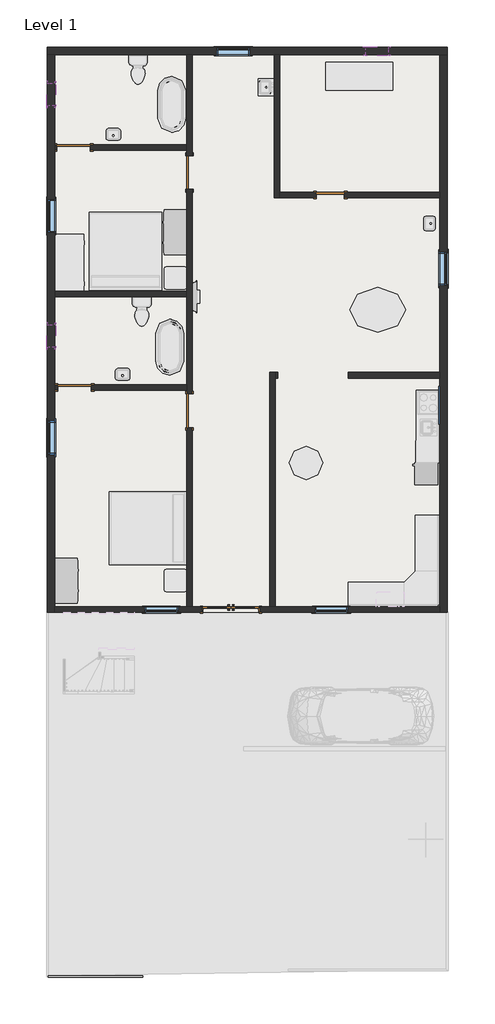
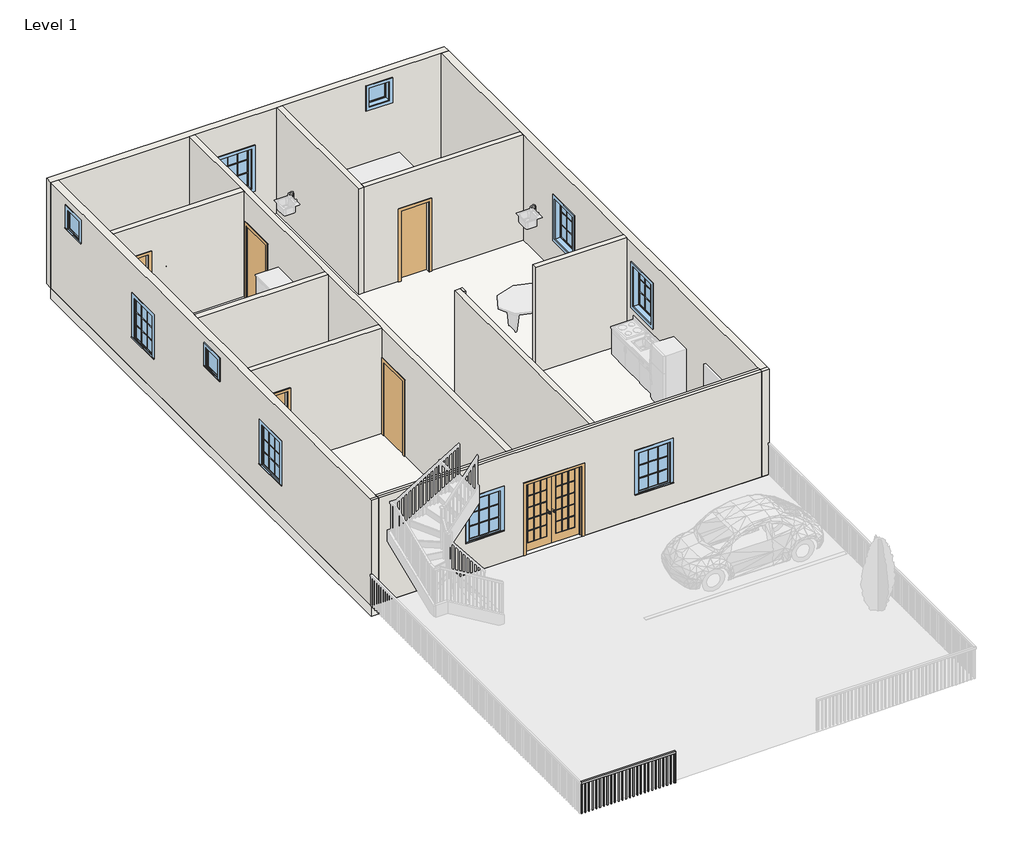
# One storey, part 1 of 5: 13 walls, 10 windows, 6 doors, 1 railing, 1 slab.
"""IFC4 building model written with IfcOpenShell, lengths in millimetres."""

from ifc_helpers import new_model, si_unit, frame, origin, origin_with_axes, place, context, project, spatial, polyline, outline, extrude, faceted_brep, transform, mapped, element, save
from components import door_31a77bde, door_255cab33, door_686f89d2, door_16372e1c, window_29c06734, window_5c190c7e, window_e41d21a6

model = new_model("IFC4")

# Units and contexts
model_context = context("Model", 3, world=origin())
ifc_project = project(units=[si_unit("LENGTHUNIT", "METRE", prefix="MILLI")], contexts=[model_context])

# Site, building, storey
site = spatial("IfcSite", under=ifc_project)
building = spatial("IfcBuilding", under=site)
storey = spatial("IfcBuildingStorey", under=building, Name="Level 1", Elevation=0.0)

# Doors
placement = place(None, origin())
door_shape = door_31a77bde(model_context)
element("IfcDoor", 1, ObjectType="Door-Interior-Double-Full Glass-Wood : 60\" x 80\"", at=placement, inside=storey, context=model_context, shape_type="MappedRepresentation", body=[
    mapped(door_shape, transform((-4021.3170266, -2394.0326646, 0.0), x_axis=(1.0, 0.0, 0.0), y_axis=(0.0, 1.0, 0.0), z_axis=(0.0, 0.0, 1.0))),
])
door_2_shape = door_255cab33(model_context)
element("IfcDoor", 2, ObjectType="Single-Flush : 30\" x 80\"", at=placement, inside=storey, context=model_context, shape_type="MappedRepresentation", body=[
    mapped(door_2_shape, transform((-1316.2170266, 8880.3923354, 0.0), x_axis=(-1.0, 0.0, 0.0), y_axis=(0.0, -1.0, 0.0), z_axis=(0.0, 0.0, 1.0))),
])
door_3_shape = door_686f89d2(model_context)
element("IfcDoor", 3, ObjectType="Single-Flush : 36\" x 84\"", at=placement, inside=storey, context=model_context, shape_type="MappedRepresentation", body=[
    mapped(door_3_shape, transform((-8301.2170266, 10175.7923354, 0.0), x_axis=(-1.0, 0.0, 0.0), y_axis=(0.0, -1.0, 0.0), z_axis=(0.0, 0.0, 1.0))),
])
element("IfcDoor", 4, ObjectType="Single-Flush : 36\" x 84\"", at=placement, inside=storey, context=model_context, shape_type="MappedRepresentation", body=[
    mapped(door_3_shape, transform((-8275.8170266, 3647.9923354, 0.0), x_axis=(-1.0, 0.0, 0.0), y_axis=(0.0, -1.0, 0.0), z_axis=(0.0, 0.0, 1.0))),
])
door_4_shape = door_16372e1c(model_context)
element("IfcDoor", 5, ObjectType="Single-Flush : 36\" x 84\"", at=placement, inside=storey, context=model_context, shape_type="MappedRepresentation", body=[
    mapped(door_4_shape, transform((-5151.6170266, 9489.9923354, 0.0), x_axis=(0.0, 1.0, 0.0), y_axis=(-1.0, 0.0, 0.0), z_axis=(0.0, 0.0, 1.0))),
])
element("IfcDoor", 6, ObjectType="Single-Flush : 36\" x 84\"", at=placement, inside=storey, context=model_context, shape_type="MappedRepresentation", body=[
    mapped(door_4_shape, transform((-5151.6170266, 3012.9923354, 0.0), x_axis=(0.0, 1.0, 0.0), y_axis=(-1.0, 0.0, 0.0), z_axis=(0.0, 0.0, 1.0))),
])

# Railing
element("IfcRailing", 7, ObjectType="Handrail - Rectangular", at=placement, inside=storey, context=model_context, shape_type="SweptSolid", body=[
    extrude(outline(polyline([(-8987.0170266, -12404.8076646), (-8987.0170266, -12354.0076646), (-6421.6170266, -12354.0076646), (-6421.6170266, -12404.8076646), (-8987.0170266, -12404.8076646)])), frame((0.0, 0.0, 863.6), z_axis=(0.0, 0.0, 1.0), x_axis=(1.0, 0.0, 0.0)), (0.0, 0.0, 1.0), 50.8),
    extrude(outline(polyline([(-6456.5420266, -12388.9326646), (-6456.5420266, -12369.8826646), (-6437.4920266, -12369.8826646), (-6437.4920266, -12388.9326646), (-6456.5420266, -12388.9326646)])), origin_with_axes(), (0.0, 0.0, 1.0), 863.6),
    extrude(outline(polyline([(-6558.1420266, -12388.9326646), (-6558.1420266, -12369.8826646), (-6539.0920266, -12369.8826646), (-6539.0920266, -12388.9326646), (-6558.1420266, -12388.9326646)])), origin_with_axes(), (0.0, 0.0, 1.0), 863.6),
    extrude(outline(polyline([(-6659.7420266, -12388.9326646), (-6659.7420266, -12369.8826646), (-6640.6920266, -12369.8826646), (-6640.6920266, -12388.9326646), (-6659.7420266, -12388.9326646)])), origin_with_axes(), (0.0, 0.0, 1.0), 863.6),
    extrude(outline(polyline([(-6761.3420266, -12388.9326646), (-6761.3420266, -12369.8826646), (-6742.2920266, -12369.8826646), (-6742.2920266, -12388.9326646), (-6761.3420266, -12388.9326646)])), origin_with_axes(), (0.0, 0.0, 1.0), 863.6),
    extrude(outline(polyline([(-6862.9420266, -12388.9326646), (-6862.9420266, -12369.8826646), (-6843.8920266, -12369.8826646), (-6843.8920266, -12388.9326646), (-6862.9420266, -12388.9326646)])), origin_with_axes(), (0.0, 0.0, 1.0), 863.6),
    extrude(outline(polyline([(-6964.5420266, -12388.9326646), (-6964.5420266, -12369.8826646), (-6945.4920266, -12369.8826646), (-6945.4920266, -12388.9326646), (-6964.5420266, -12388.9326646)])), origin_with_axes(), (0.0, 0.0, 1.0), 863.6),
    extrude(outline(polyline([(-7066.1420266, -12388.9326646), (-7066.1420266, -12369.8826646), (-7047.0920266, -12369.8826646), (-7047.0920266, -12388.9326646), (-7066.1420266, -12388.9326646)])), origin_with_axes(), (0.0, 0.0, 1.0), 863.6),
    extrude(outline(polyline([(-7167.7420266, -12388.9326646), (-7167.7420266, -12369.8826646), (-7148.6920266, -12369.8826646), (-7148.6920266, -12388.9326646), (-7167.7420266, -12388.9326646)])), origin_with_axes(), (0.0, 0.0, 1.0), 863.6),
    extrude(outline(polyline([(-7269.3420266, -12388.9326646), (-7269.3420266, -12369.8826646), (-7250.2920266, -12369.8826646), (-7250.2920266, -12388.9326646), (-7269.3420266, -12388.9326646)])), origin_with_axes(), (0.0, 0.0, 1.0), 863.6),
    extrude(outline(polyline([(-7370.9420266, -12388.9326646), (-7370.9420266, -12369.8826646), (-7351.8920266, -12369.8826646), (-7351.8920266, -12388.9326646), (-7370.9420266, -12388.9326646)])), origin_with_axes(), (0.0, 0.0, 1.0), 863.6),
    extrude(outline(polyline([(-7472.5420266, -12388.9326646), (-7472.5420266, -12369.8826646), (-7453.4920266, -12369.8826646), (-7453.4920266, -12388.9326646), (-7472.5420266, -12388.9326646)])), origin_with_axes(), (0.0, 0.0, 1.0), 863.6),
    extrude(outline(polyline([(-7574.1420266, -12388.9326646), (-7574.1420266, -12369.8826646), (-7555.0920266, -12369.8826646), (-7555.0920266, -12388.9326646), (-7574.1420266, -12388.9326646)])), origin_with_axes(), (0.0, 0.0, 1.0), 863.6),
    extrude(outline(polyline([(-7675.7420266, -12388.9326646), (-7675.7420266, -12369.8826646), (-7656.6920266, -12369.8826646), (-7656.6920266, -12388.9326646), (-7675.7420266, -12388.9326646)])), origin_with_axes(), (0.0, 0.0, 1.0), 863.6),
    extrude(outline(polyline([(-7777.3420266, -12388.9326646), (-7777.3420266, -12369.8826646), (-7758.2920266, -12369.8826646), (-7758.2920266, -12388.9326646), (-7777.3420266, -12388.9326646)])), origin_with_axes(), (0.0, 0.0, 1.0), 863.6),
    extrude(outline(polyline([(-7878.9420266, -12388.9326646), (-7878.9420266, -12369.8826646), (-7859.8920266, -12369.8826646), (-7859.8920266, -12388.9326646), (-7878.9420266, -12388.9326646)])), origin_with_axes(), (0.0, 0.0, 1.0), 863.6),
    extrude(outline(polyline([(-7980.5420266, -12388.9326646), (-7980.5420266, -12369.8826646), (-7961.4920266, -12369.8826646), (-7961.4920266, -12388.9326646), (-7980.5420266, -12388.9326646)])), origin_with_axes(), (0.0, 0.0, 1.0), 863.6),
    extrude(outline(polyline([(-8082.1420266, -12388.9326646), (-8082.1420266, -12369.8826646), (-8063.0920266, -12369.8826646), (-8063.0920266, -12388.9326646), (-8082.1420266, -12388.9326646)])), origin_with_axes(), (0.0, 0.0, 1.0), 863.6),
    extrude(outline(polyline([(-8183.7420266, -12388.9326646), (-8183.7420266, -12369.8826646), (-8164.6920266, -12369.8826646), (-8164.6920266, -12388.9326646), (-8183.7420266, -12388.9326646)])), origin_with_axes(), (0.0, 0.0, 1.0), 863.6),
    extrude(outline(polyline([(-8285.3420266, -12388.9326646), (-8285.3420266, -12369.8826646), (-8266.2920266, -12369.8826646), (-8266.2920266, -12388.9326646), (-8285.3420266, -12388.9326646)])), origin_with_axes(), (0.0, 0.0, 1.0), 863.6),
    extrude(outline(polyline([(-8386.9420266, -12388.9326646), (-8386.9420266, -12369.8826646), (-8367.8920266, -12369.8826646), (-8367.8920266, -12388.9326646), (-8386.9420266, -12388.9326646)])), origin_with_axes(), (0.0, 0.0, 1.0), 863.6),
    extrude(outline(polyline([(-8488.5420266, -12388.9326646), (-8488.5420266, -12369.8826646), (-8469.4920266, -12369.8826646), (-8469.4920266, -12388.9326646), (-8488.5420266, -12388.9326646)])), origin_with_axes(), (0.0, 0.0, 1.0), 863.6),
    extrude(outline(polyline([(-8590.1420266, -12388.9326646), (-8590.1420266, -12369.8826646), (-8571.0920266, -12369.8826646), (-8571.0920266, -12388.9326646), (-8590.1420266, -12388.9326646)])), origin_with_axes(), (0.0, 0.0, 1.0), 863.6),
    extrude(outline(polyline([(-8691.7420266, -12388.9326646), (-8691.7420266, -12369.8826646), (-8672.6920266, -12369.8826646), (-8672.6920266, -12388.9326646), (-8691.7420266, -12388.9326646)])), origin_with_axes(), (0.0, 0.0, 1.0), 863.6),
    extrude(outline(polyline([(-8793.3420266, -12388.9326646), (-8793.3420266, -12369.8826646), (-8774.2920266, -12369.8826646), (-8774.2920266, -12388.9326646), (-8793.3420266, -12388.9326646)])), origin_with_axes(), (0.0, 0.0, 1.0), 863.6),
    extrude(outline(polyline([(-8894.9420266, -12388.9326646), (-8894.9420266, -12369.8826646), (-8875.8920266, -12369.8826646), (-8875.8920266, -12388.9326646), (-8894.9420266, -12388.9326646)])), origin_with_axes(), (0.0, 0.0, 1.0), 863.6),
    extrude(outline(polyline([(-6440.6670266, -12388.9326646), (-6440.6670266, -12369.8826646), (-6421.6170266, -12369.8826646), (-6421.6170266, -12388.9326646), (-6440.6670266, -12388.9326646)])), origin_with_axes(), (0.0, 0.0, 1.0), 863.6),
    extrude(outline(polyline([(-8987.0170266, -12388.9326646), (-8987.0170266, -12369.8826646), (-8967.9670266, -12369.8826646), (-8967.9670266, -12388.9326646), (-8987.0170266, -12388.9326646)])), origin_with_axes(), (0.0, 0.0, 1.0), 863.6),
])

# Slab
element("IfcSlab", 8, ObjectType="Generic - 12\"", at=placement, inside=storey, context=model_context, shape_type="SweptSolid", body=[
    extrude(outline(polyline([(1858.7829734, 12690.3923354), (1858.7829734, -2473.4076646), (-9012.4170266, -2473.4076646), (-9012.4170266, 12690.3923354), (1858.7829734, 12690.3923354)])), frame((0.0, 0.0, -304.8), z_axis=(0.0, 0.0, 1.0), x_axis=(1.0, 0.0, 0.0)), (0.0, 0.0, 1.0), 304.8),
])

# Walls
element("IfcWall", 9, ObjectType="Generic - 8\"", at=placement, inside=storey, context=model_context, shape_type="Brep", body=[
    faceted_brep([(-9012.4170266, 12690.3923354, 0.0), (-8809.2170266, 12690.3923354, 0.0), (-5227.8170266, 12690.3923354, 0.0), (-5075.4170266, 12690.3923354, 0.0), (-2840.2170266, 12690.3923354, 0.0), (-2687.8170266, 12690.3923354, 0.0), (1655.5829734, 12690.3923354, 0.0), (1858.7829734, 12690.3923354, 0.0), (1858.7829734, 12690.3923354, 3048.0), (1655.5829734, 12690.3923354, 3048.0), (-2687.8170266, 12690.3923354, 3048.0), (-2840.2170266, 12690.3923354, 3048.0), (-5075.4170266, 12690.3923354, 3048.0), (-5227.8170266, 12690.3923354, 3048.0), (-8809.2170266, 12690.3923354, 3048.0), (-9012.4170266, 12690.3923354, 3048.0), (-3500.6170266, 12690.3923354, 2133.6), (-3500.6170266, 12690.3923354, 914.4), (-4415.0170266, 12690.3923354, 914.4), (-4415.0170266, 12690.3923354, 2133.6), (258.5829734, 12690.3923354, 2768.6), (258.5829734, 12690.3923354, 2159.0), (-351.0170266, 12690.3923354, 2159.0), (-351.0170266, 12690.3923354, 2768.6), (-9012.4170266, 12893.5923354, 0.0), (-9012.4170266, 12893.5923354, 3048.0), (1858.7829734, 12893.5923354, 3048.0), (1858.7829734, 12893.5923354, 0.0), (-3500.6170266, 12893.5923354, 2133.6), (-4415.0170266, 12893.5923354, 2133.6), (-4415.0170266, 12893.5923354, 914.4), (-3500.6170266, 12893.5923354, 914.4), (258.5829734, 12893.5923354, 2768.6), (-351.0170266, 12893.5923354, 2768.6), (-351.0170266, 12893.5923354, 2159.0), (258.5829734, 12893.5923354, 2159.0)], [[[0, 1, 2, 3, 4, 5, 6, 7, 8, 9, 10, 11, 12, 13, 14, 15], [16, 17, 18, 19], [20, 21, 22, 23]], [[24, 25, 26, 27], [28, 29, 30, 31], [32, 33, 34, 35]], [[7, 6, 5, 4, 3, 2, 1, 0, 24, 27]], [[0, 15, 25, 24]], [[8, 7, 27, 26]], [[17, 16, 28, 31]], [[18, 17, 31, 30]], [[19, 18, 30, 29]], [[16, 19, 29, 28]], [[21, 20, 32, 35]], [[22, 21, 35, 34]], [[23, 22, 34, 33]], [[20, 23, 33, 32]], [[15, 14, 13, 12, 11, 10, 9, 8, 26, 25]]]),
])
element("IfcWall", 10, ObjectType="Generic - 8\"", at=placement, inside=storey, context=model_context, shape_type="Brep", body=[
    faceted_brep([(-9012.4170266, 12690.3923354, 0.0), (-9012.4170266, -2473.4076646, 0.0), (-9012.4170266, -2473.4076646, 3048.0), (-9012.4170266, -2397.2076646, 3048.0), (-9012.4170266, 12690.3923354, 3048.0), (-9012.4170266, 8766.0923354, 2133.6), (-9012.4170266, 7851.6923354, 2133.6), (-9012.4170266, 7851.6923354, 914.4), (-9012.4170266, 8766.0923354, 914.4), (-9012.4170266, 2733.5923354, 2133.6), (-9012.4170266, 1819.1923354, 2133.6), (-9012.4170266, 1819.1923354, 914.4), (-9012.4170266, 2733.5923354, 914.4), (-9012.4170266, 11915.6923354, 2768.6), (-9012.4170266, 11306.0923354, 2768.6), (-9012.4170266, 11306.0923354, 2159.0), (-9012.4170266, 11915.6923354, 2159.0), (-9012.4170266, 5349.7923354, 2768.6), (-9012.4170266, 4740.1923354, 2768.6), (-9012.4170266, 4740.1923354, 2159.0), (-9012.4170266, 5349.7923354, 2159.0), (-8809.2170266, 12690.3923354, 0.0), (-8809.2170266, 12690.3923354, 3048.0), (-8809.2170266, 10251.9923354, 3048.0), (-8809.2170266, 10099.5923354, 3048.0), (-8809.2170266, 6264.1923354, 3048.0), (-8809.2170266, 6111.7923354, 3048.0), (-8809.2170266, 3724.1923354, 3048.0), (-8809.2170266, 3571.7923354, 3048.0), (-8809.2170266, -2321.0076646, 3048.0), (-8809.2170266, -2397.2076646, 3048.0), (-8809.2170266, -2473.4076646, 3048.0), (-8809.2170266, -2473.4076646, 0.0), (-8809.2170266, -2321.0076646, 0.0), (-8809.2170266, 3571.7923354, 0.0), (-8809.2170266, 3724.1923354, 0.0), (-8809.2170266, 6111.7923354, 0.0), (-8809.2170266, 6264.1923354, 0.0), (-8809.2170266, 10099.5923354, 0.0), (-8809.2170266, 10251.9923354, 0.0), (-8809.2170266, 8766.0923354, 2133.6), (-8809.2170266, 8766.0923354, 914.4), (-8809.2170266, 7851.6923354, 914.4), (-8809.2170266, 7851.6923354, 2133.6), (-8809.2170266, 2733.5923354, 2133.6), (-8809.2170266, 2733.5923354, 914.4), (-8809.2170266, 1819.1923354, 914.4), (-8809.2170266, 1819.1923354, 2133.6), (-8809.2170266, 11915.6923354, 2768.6), (-8809.2170266, 11915.6923354, 2159.0), (-8809.2170266, 11306.0923354, 2159.0), (-8809.2170266, 11306.0923354, 2768.6), (-8809.2170266, 5349.7923354, 2768.6), (-8809.2170266, 5349.7923354, 2159.0), (-8809.2170266, 4740.1923354, 2159.0), (-8809.2170266, 4740.1923354, 2768.6)], [[[0, 1, 2, 3, 4], [5, 6, 7, 8], [9, 10, 11, 12], [13, 14, 15, 16], [17, 18, 19, 20]], [[21, 22, 23, 24, 25, 26, 27, 28, 29, 30, 31, 32, 33, 34, 35, 36, 37, 38, 39], [40, 41, 42, 43], [44, 45, 46, 47], [48, 49, 50, 51], [52, 53, 54, 55]], [[1, 0, 21, 39, 38, 37, 36, 35, 34, 33, 32]], [[0, 4, 22, 21]], [[41, 40, 5, 8]], [[42, 41, 8, 7]], [[43, 42, 7, 6]], [[40, 43, 6, 5]], [[45, 44, 9, 12]], [[46, 45, 12, 11]], [[47, 46, 11, 10]], [[44, 47, 10, 9]], [[49, 48, 13, 16]], [[50, 49, 16, 15]], [[51, 50, 15, 14]], [[48, 51, 14, 13]], [[53, 52, 17, 20]], [[54, 53, 20, 19]], [[55, 54, 19, 18]], [[52, 55, 18, 17]], [[2, 1, 32, 31]], [[3, 2, 31, 30]], [[4, 3, 30, 29, 28, 27, 26, 25, 24, 23, 22]]]),
])
element("IfcWall", 11, ObjectType="Generic - 8\"", at=placement, inside=storey, context=model_context, shape_type="Brep", body=[
    faceted_brep([(1858.7829734, -2473.4076646, 0.0), (1858.7829734, 12690.3923354, 0.0), (1858.7829734, 12690.3923354, 3048.0), (1858.7829734, -2397.2076646, 3048.0), (1858.7829734, -2473.4076646, 3048.0), (1858.7829734, 2708.1923354, 2438.4), (1858.7829734, 3622.5923354, 2438.4), (1858.7829734, 3622.5923354, 1219.2), (1858.7829734, 2708.1923354, 1219.2), (1858.7829734, 6416.5923354, 2133.6), (1858.7829734, 7330.9923354, 2133.6), (1858.7829734, 7330.9923354, 914.4), (1858.7829734, 6416.5923354, 914.4), (1655.5829734, -2473.4076646, 0.0), (1655.5829734, -2473.4076646, 3048.0), (1655.5829734, -2397.2076646, 3048.0), (1655.5829734, -2321.0076646, 3048.0), (1655.5829734, 3901.9923354, 3048.0), (1655.5829734, 4054.3923354, 3048.0), (1655.5829734, 8804.1923354, 3048.0), (1655.5829734, 8956.5923354, 3048.0), (1655.5829734, 12690.3923354, 3048.0), (1655.5829734, 12690.3923354, 0.0), (1655.5829734, 8956.5923354, 0.0), (1655.5829734, 8804.1923354, 0.0), (1655.5829734, 4054.3923354, 0.0), (1655.5829734, 3901.9923354, 0.0), (1655.5829734, -2321.0076646, 0.0), (1655.5829734, 2708.1923354, 2438.4), (1655.5829734, 2708.1923354, 1219.2), (1655.5829734, 3622.5923354, 1219.2), (1655.5829734, 3622.5923354, 2438.4), (1655.5829734, 6416.5923354, 2133.6), (1655.5829734, 6416.5923354, 914.4), (1655.5829734, 7330.9923354, 914.4), (1655.5829734, 7330.9923354, 2133.6)], [[[0, 1, 2, 3, 4], [5, 6, 7, 8], [9, 10, 11, 12]], [[13, 14, 15, 16, 17, 18, 19, 20, 21, 22, 23, 24, 25, 26, 27], [28, 29, 30, 31], [32, 33, 34, 35]], [[1, 0, 13, 27, 26, 25, 24, 23, 22]], [[2, 1, 22, 21]], [[28, 31, 6, 5]], [[31, 30, 7, 6]], [[30, 29, 8, 7]], [[29, 28, 5, 8]], [[32, 35, 10, 9]], [[35, 34, 11, 10]], [[34, 33, 12, 11]], [[33, 32, 9, 12]], [[0, 4, 14, 13]], [[4, 3, 15, 14]], [[3, 2, 21, 20, 19, 18, 17, 16, 15]]]),
])
element("IfcWall", 12, ObjectType="INNER WALL 6\"", at=placement, inside=storey, context=model_context, shape_type="Brep", body=[
    faceted_brep([(-5227.8170266, 9032.7923354, 0.0), (-5227.8170266, 6264.1923354, 0.0), (-5227.8170266, 6111.7923354, 0.0), (-5227.8170266, 3724.1923354, 0.0), (-5227.8170266, 3571.7923354, 0.0), (-5227.8170266, 3470.1923354, 0.0), (-5227.8170266, 3470.1923354, 2133.6), (-5227.8170266, 2555.7923354, 2133.6), (-5227.8170266, 2555.7923354, 0.0), (-5227.8170266, -2321.0076646, 0.0), (-5227.8170266, -2321.0076646, 3048.0), (-5227.8170266, 3571.7923354, 3048.0), (-5227.8170266, 3724.1923354, 3048.0), (-5227.8170266, 6111.7923354, 3048.0), (-5227.8170266, 6264.1923354, 3048.0), (-5227.8170266, 10099.5923354, 3048.0), (-5227.8170266, 10251.9923354, 3048.0), (-5227.8170266, 12690.3923354, 3048.0), (-5227.8170266, 12690.3923354, 0.0), (-5227.8170266, 10251.9923354, 0.0), (-5227.8170266, 10099.5923354, 0.0), (-5227.8170266, 9947.1923354, 0.0), (-5227.8170266, 9947.1923354, 2133.6), (-5227.8170266, 9032.7923354, 2133.6), (-5075.4170266, 3470.1923354, 2133.6), (-5075.4170266, 3470.1923354, 0.0), (-5075.4170266, 9032.7923354, 0.0), (-5075.4170266, 9032.7923354, 2133.6), (-5075.4170266, 9947.1923354, 2133.6), (-5075.4170266, 9947.1923354, 0.0), (-5075.4170266, 12690.3923354, 0.0), (-5075.4170266, 12690.3923354, 3048.0), (-5075.4170266, -2321.0076646, 3048.0), (-5075.4170266, -2321.0076646, 0.0), (-5075.4170266, 2555.7923354, 0.0), (-5075.4170266, 2555.7923354, 2133.6)], [[[0, 1, 2, 3, 4, 5, 6, 7, 8, 9, 10, 11, 12, 13, 14, 15, 16, 17, 18, 19, 20, 21, 22, 23]], [[24, 25, 26, 27, 28, 29, 30, 31, 32, 33, 34, 35]], [[30, 29, 21, 20, 19, 18]], [[34, 33, 9, 8]], [[26, 25, 5, 4, 3, 2, 1, 0]], [[18, 17, 31, 30]], [[10, 9, 33, 32]], [[22, 21, 29, 28]], [[23, 22, 28, 27]], [[0, 23, 27, 26]], [[6, 5, 25, 24]], [[7, 6, 24, 35]], [[8, 7, 35, 34]], [[17, 16, 15, 14, 13, 12, 11, 10, 32, 31]]]),
])
element("IfcWall", 13, ObjectType="INNER WALL 6\"", at=placement, inside=storey, context=model_context, shape_type="Brep", body=[
    faceted_brep([(1655.5829734, -2321.0076646, 3048.0), (1655.5829734, -2321.0076646, 0.0), (-2814.8170266, -2321.0076646, 0.0), (-2967.2170266, -2321.0076646, 0.0), (-3233.9170266, -2321.0076646, 0.0), (-3233.9170266, -2321.0076646, 2057.4), (-4808.7170266, -2321.0076646, 2057.4), (-4808.7170266, -2321.0076646, 0.0), (-5075.4170266, -2321.0076646, 0.0), (-5227.8170266, -2321.0076646, 0.0), (-8809.2170266, -2321.0076646, 0.0), (-8809.2170266, -2321.0076646, 3048.0), (-5227.8170266, -2321.0076646, 3048.0), (-5075.4170266, -2321.0076646, 3048.0), (-2967.2170266, -2321.0076646, 3048.0), (-2814.8170266, -2321.0076646, 3048.0), (-6370.8170266, -2321.0076646, 2133.6), (-6370.8170266, -2321.0076646, 914.4), (-5456.4170266, -2321.0076646, 914.4), (-5456.4170266, -2321.0076646, 2133.6), (-1748.0170266, -2321.0076646, 1905.0), (-1748.0170266, -2321.0076646, 685.8), (-833.6170266, -2321.0076646, 685.8), (-833.6170266, -2321.0076646, 1905.0), (1655.5829734, -2473.4076646, 3048.0), (-8809.2170266, -2473.4076646, 3048.0), (-8809.2170266, -2473.4076646, 0.0), (-4808.7170266, -2473.4076646, 0.0), (-4808.7170266, -2473.4076646, 2057.4), (-3233.9170266, -2473.4076646, 2057.4), (-3233.9170266, -2473.4076646, 0.0), (1655.5829734, -2473.4076646, 0.0), (-6370.8170266, -2473.4076646, 2133.6), (-5456.4170266, -2473.4076646, 2133.6), (-5456.4170266, -2473.4076646, 914.4), (-6370.8170266, -2473.4076646, 914.4), (-1748.0170266, -2473.4076646, 1905.0), (-833.6170266, -2473.4076646, 1905.0), (-833.6170266, -2473.4076646, 685.8), (-1748.0170266, -2473.4076646, 685.8), (1655.5829734, -2397.2076646, 3048.0), (-8809.2170266, -2397.2076646, 3048.0)], [[[0, 1, 2, 3, 4, 5, 6, 7, 8, 9, 10, 11, 12, 13, 14, 15], [16, 17, 18, 19], [20, 21, 22, 23]], [[24, 25, 26, 27, 28, 29, 30, 31], [32, 33, 34, 35], [36, 37, 38, 39]], [[1, 31, 30, 4, 3, 2]], [[26, 10, 9, 8, 7, 27]], [[29, 5, 4, 30]], [[5, 29, 28, 6]], [[6, 28, 27, 7]], [[17, 16, 32, 35]], [[18, 17, 35, 34]], [[19, 18, 34, 33]], [[16, 19, 33, 32]], [[21, 20, 36, 39]], [[22, 21, 39, 38]], [[23, 22, 38, 37]], [[20, 23, 37, 36]], [[1, 0, 40, 24, 31]], [[11, 10, 26, 25, 41]], [[25, 24, 40, 41]], [[0, 15, 14, 13, 12, 11, 41, 40]]]),
])
element("IfcWall", 14, ObjectType="INNER WALL 6\"", at=placement, inside=storey, context=model_context, shape_type="Brep", body=[
    faceted_brep([(-2814.8170266, -2321.0076646, 0.0), (-2814.8170266, 3901.9923354, 0.0), (-2814.8170266, 4054.3923354, 0.0), (-2814.8170266, 4054.3923354, 3048.0), (-2814.8170266, 3901.9923354, 3048.0), (-2814.8170266, -2321.0076646, 3048.0), (-2967.2170266, -2321.0076646, 0.0), (-2967.2170266, -2321.0076646, 3048.0), (-2967.2170266, 4054.3923354, 3048.0), (-2967.2170266, 4054.3923354, 0.0)], [[[0, 1, 2, 3, 4, 5]], [[6, 7, 8, 9]], [[2, 1, 0, 6, 9]], [[0, 5, 7, 6]], [[3, 2, 9, 8]], [[5, 4, 3, 8, 7]]]),
])
element("IfcWall", 15, ObjectType="INNER WALL 6\"", at=placement, inside=storey, context=model_context, shape_type="SweptSolid", body=[
    extrude(outline(polyline([(-2751.3170266, 3901.9923354), (-2814.8170266, 3901.9923354), (-2814.8170266, 4054.3923354), (-2751.3170266, 4054.3923354), (-2751.3170266, 3901.9923354)])), origin_with_axes(), (0.0, 0.0, 1.0), 3048.0),
])
element("IfcWall", 16, ObjectType="INNER WALL 6\"", at=placement, inside=storey, context=model_context, shape_type="Brep", body=[
    faceted_brep([(-2840.2170266, 12690.3923354, 0.0), (-2840.2170266, 8804.1923354, 0.0), (-2840.2170266, 8804.1923354, 3048.0), (-2840.2170266, 12690.3923354, 3048.0), (-2687.8170266, 12690.3923354, 0.0), (-2687.8170266, 12690.3923354, 3048.0), (-2687.8170266, 8956.5923354, 3048.0), (-2687.8170266, 8804.1923354, 3048.0), (-2687.8170266, 8804.1923354, 0.0), (-2687.8170266, 8956.5923354, 0.0)], [[[0, 1, 2, 3]], [[4, 5, 6, 7, 8, 9]], [[1, 0, 4, 9, 8]], [[0, 3, 5, 4]], [[2, 1, 8, 7]], [[3, 2, 7, 6, 5]]]),
])
element("IfcWall", 17, ObjectType="INNER WALL 6\"", at=placement, inside=storey, context=model_context, shape_type="SweptSolid", body=[
    extrude(outline(polyline([(0.0, -2687.8170266), (0.0, -1697.2170266), (2032.0, -1697.2170266), (2032.0, -935.2170266), (0.0, -935.2170266), (0.0, 1655.5829734), (3048.0, 1655.5829734), (3048.0, -2687.8170266), (0.0, -2687.8170266)])), frame((0.0, 8804.1923354, 0.0), z_axis=(0.0, 1.0, 0.0), x_axis=(0.0, 0.0, 1.0)), (0.0, 0.0, 1.0), 152.4),
])
element("IfcWall", 18, ObjectType="INNER WALL 6\"", at=placement, inside=storey, context=model_context, shape_type="SweptSolid", body=[
    extrude(outline(polyline([(0.0, -8809.2170266), (0.0, -8758.4170266), (2133.6, -8758.4170266), (2133.6, -7844.0170266), (0.0, -7844.0170266), (0.0, -5227.8170266), (3048.0, -5227.8170266), (3048.0, -8809.2170266), (0.0, -8809.2170266)])), frame((0.0, 10099.5923354, 0.0), z_axis=(0.0, 1.0, 0.0), x_axis=(0.0, 0.0, 1.0)), (0.0, 0.0, 1.0), 152.4),
])
element("IfcWall", 19, ObjectType="INNER WALL 6\"", at=placement, inside=storey, context=model_context, shape_type="SweptSolid", body=[
    extrude(outline(polyline([(-5227.8170266, 6111.7923354), (-8809.2170266, 6111.7923354), (-8809.2170266, 6264.1923354), (-5227.8170266, 6264.1923354), (-5227.8170266, 6111.7923354)])), origin_with_axes(), (0.0, 0.0, 1.0), 3048.0),
])
element("IfcWall", 20, ObjectType="INNER WALL 6\"", at=placement, inside=storey, context=model_context, shape_type="SweptSolid", body=[
    extrude(outline(polyline([(0.0, -8809.2170266), (0.0, -8733.0170266), (2133.6, -8733.0170266), (2133.6, -7818.6170266), (0.0, -7818.6170266), (0.0, -5227.8170266), (3048.0, -5227.8170266), (3048.0, -8809.2170266), (0.0, -8809.2170266)])), frame((0.0, 3571.7923354, 0.0), z_axis=(0.0, 1.0, 0.0), x_axis=(0.0, 0.0, 1.0)), (0.0, 0.0, 1.0), 152.4),
])
element("IfcWall", 21, ObjectType="INNER WALL 6\"", at=placement, inside=storey, context=model_context, shape_type="SweptSolid", body=[
    extrude(outline(polyline([(1655.5829734, 3901.9923354), (-833.6170266, 3901.9923354), (-833.6170266, 4054.3923354), (1655.5829734, 4054.3923354), (1655.5829734, 3901.9923354)])), origin_with_axes(), (0.0, 0.0, 1.0), 3048.0),
])

# Windows
window_shape = window_29c06734(model_context)
element("IfcWindow", 22, ObjectType="Casement 3x3 with Trim : 36\" x 48\"", at=placement, inside=storey, context=model_context, shape_type="MappedRepresentation", body=[
    mapped(window_shape, transform((-8910.8170266, 8308.8923354, 0.0), x_axis=(0.0, 1.0, 0.0), y_axis=(-1.0, 0.0, 0.0), z_axis=(0.0, 0.0, 1.0))),
])
element("IfcWindow", 23, ObjectType="Casement 3x3 with Trim : 36\" x 48\"", at=placement, inside=storey, context=model_context, shape_type="MappedRepresentation", body=[
    mapped(window_shape, transform((-8910.8170266, 2276.3923354, 0.0), x_axis=(0.0, 1.0, 0.0), y_axis=(-1.0, 0.0, 0.0), z_axis=(0.0, 0.0, 1.0))),
])
element("IfcWindow", 24, ObjectType="Casement 3x3 with Trim : 36\" x 48\"", at=placement, inside=storey, context=model_context, shape_type="MappedRepresentation", body=[
    mapped(window_shape, transform((1757.1829734, 3165.3923354, 304.8), x_axis=(0.0, -1.0, 0.0), y_axis=(1.0, 0.0, 0.0), z_axis=(0.0, 0.0, 1.0))),
])
element("IfcWindow", 25, ObjectType="Casement 3x3 with Trim : 36\" x 48\"", at=placement, inside=storey, context=model_context, shape_type="MappedRepresentation", body=[
    mapped(window_shape, transform((1757.1829734, 6873.7923354, 0.0), x_axis=(0.0, -1.0, 0.0), y_axis=(1.0, 0.0, 0.0), z_axis=(0.0, 0.0, 1.0))),
])
element("IfcWindow", 26, ObjectType="Casement 3x3 with Trim : 36\" x 48\"", at=placement, inside=storey, context=model_context, shape_type="MappedRepresentation", body=[
    mapped(window_shape, transform((-3957.8170266, 12791.9923354, 0.0), x_axis=(1.0, 0.0, 0.0), y_axis=(0.0, 1.0, 0.0), z_axis=(0.0, 0.0, 1.0))),
])
window_2_shape = window_5c190c7e(model_context)
element("IfcWindow", 27, ObjectType="Casement 3x3 with Trim : 36\" x 48\"", at=placement, inside=storey, context=model_context, shape_type="MappedRepresentation", body=[
    mapped(window_2_shape, transform((-5913.6170266, -2397.2076646, 0.0), x_axis=(-1.0, 0.0, 0.0), y_axis=(0.0, -1.0, 0.0), z_axis=(0.0, 0.0, 1.0))),
])
element("IfcWindow", 28, ObjectType="Casement 3x3 with Trim : 36\" x 48\"", at=placement, inside=storey, context=model_context, shape_type="MappedRepresentation", body=[
    mapped(window_2_shape, transform((-1290.8170266, -2397.2076646, -228.6), x_axis=(-1.0, 0.0, 0.0), y_axis=(0.0, -1.0, 0.0), z_axis=(0.0, 0.0, 1.0))),
])
window_3_shape = window_e41d21a6(model_context)
element("IfcWindow", 29, ObjectType="Transom with Trim : 24\" x 24\"", at=placement, inside=storey, context=model_context, shape_type="MappedRepresentation", body=[
    mapped(window_3_shape, transform((-8910.8170266, 11648.9923354, 0.0), x_axis=(0.0, 1.0, 0.0), y_axis=(-1.0, 0.0, 0.0), z_axis=(0.0, 0.0, 1.0))),
])
element("IfcWindow", 30, ObjectType="Transom with Trim : 24\" x 24\"", at=placement, inside=storey, context=model_context, shape_type="MappedRepresentation", body=[
    mapped(window_3_shape, transform((-8910.8170266, 5083.0923354, 0.0), x_axis=(0.0, 1.0, 0.0), y_axis=(-1.0, 0.0, 0.0), z_axis=(0.0, 0.0, 1.0))),
])
element("IfcWindow", 31, ObjectType="Transom with Trim : 24\" x 24\"", at=placement, inside=storey, context=model_context, shape_type="MappedRepresentation", body=[
    mapped(window_3_shape, transform((-8.1170266, 12791.9923354, 0.0), x_axis=(1.0, 0.0, 0.0), y_axis=(0.0, 1.0, 0.0), z_axis=(0.0, 0.0, 1.0))),
])

save(model, "model.ifc")

# Revit data of these elements
# Type "Door-Interior-Double-Full Glass-Wood : 60\" x 80\""
#   Type Mark = "8"
#   Assembly Code = "C1020300"
#   Analytic Construction = "French door, wood frame with single glass"
#   Top Rail = 0' - 4 11/16"
#   Thickness = 0' - 1 3/8"
#   Thermal Resistance (R) = 1.0696 (h·ft²·°F)/BTU
#   Swing Angle [instance default] = 90.00°
#   Stiles = 0' - 4 3/4"
#   Rough Width = 5' - 2"
#   Rough Height = 6' - 9"
#   Panel Width = 2' - 6"
#   Height = 6' - 8"
#   Width = 5' - 0"
#   Heat Transfer Coefficient (U) = 0.9350 BTU/(h·ft²·°F)
#   Bottom Rail = 0' - 9 1/8"
#   Show Grill [instance default] = yes
#   Trim Material = Cherry
#   Panel Material = Cherry
#   Frame Material = Cherry
#   Door Handle Material = Aluminum
#   Visual Light Transmittance = 0
#   Solar Heat Gain Coefficient = 0
#   Wall Closure = (empty or 0)
#   Function = (empty or 0)
# Type "Single-Flush : 30\" x 80\""
#   Type Mark = "5"
#   Construction Type Id = "MDOOR"
#   Assembly Code = "C1020"
#   Analytic Construction = "Metal"
#   Thickness = 0' - 2"
#   Heat Transfer Coefficient (U) = 0.651978 BTU/(h·ft²·°F)
#   Height = 6' - 8"
#   Trim Projection Ext = 0' - 1"
#   Trim Projection Int = 0' - 1"
#   Trim Width = 0' - 3"
#   Width = 2' - 6"
#   Define Thermal Properties by = 1
#   Door Material = Door - Panel
#   Frame Material = Door - Frame
#   Visual Light Transmittance = 0
#   Solar Heat Gain Coefficient = 0
#   Function = (empty or 0)
#   Wall Closure = (empty or 0)
# Type "Single-Flush : 36\" x 84\""
#   Type Mark = "1"
#   Construction Type Id = "MDOOR"
#   Assembly Code = "C1020"
#   Analytic Construction = "Metal"
#   Thickness = 0' - 2"
#   Heat Transfer Coefficient (U) = 0.651978 BTU/(h·ft²·°F)
#   Height = 7' - 0"
#   Trim Projection Ext = 0' - 1"
#   Trim Projection Int = 0' - 1"
#   Trim Width = 0' - 3"
#   Width = 3' - 0"
#   Define Thermal Properties by = 1
#   Door Material = Door - Panel
#   Frame Material = Door - Frame
#   Visual Light Transmittance = 0
#   Solar Heat Gain Coefficient = 0
#   Function = (empty or 0)
#   Wall Closure = (empty or 0)
# Type "Handrail - Rectangular"
#   Assembly Code = "C2010400"
#   built-in parameter 1008612 = 0.0416667 (stored number, unit not read)
#   built-in parameter 1008611 = 0.0416667 (stored number, unit not read)
#   built-in parameter 1008609 = 0.333333 (stored number, unit not read)
#   built-in parameter 1008604 = 0.166667 (stored number, unit not read)
#   built-in parameter 1008603 = 0.166667 (stored number, unit not read)
#   Railing Height = 3' - 0"
#   built-in parameter 1008630 = 2
#   built-in parameter 1008610 = 2
#   built-in parameter 1008618 = Baluster - Square : 3/4"
# Type "Generic - 12\""
#   Assembly Code = "B1010"
#   Function = 0
#   Layers, outside or top first: 1' - 0" no material (function 1)
# Type "Generic - 8\""
#   Assembly Code = "B2010"
#   Layers, outside or top first: 0' - 8" "Brick, Common" (function 1)
# Type "INNER WALL 6\""
#   Assembly Code = "B2010"
#   Layers, outside or top first: 0' - 6" "Brick, Common" (function 1)
# Type "Casement 3x3 with Trim : 36\" x 48\""
#   Type Mark = "10"
#   Construction Type Id = "GSP4R"
#   Assembly Code = "B2020100"
#   Analytic Construction = "1/8 in Pilkington single glazing"
#   Visual Light Transmittance = 0.9
#   Solar Heat Gain Coefficient = 0.78
#   Heat Transfer Coefficient (U) = 0.6496 BTU/(h·ft²·°F)
#   Height = 4' - 0"
#   Default Sill Height = 3' - 0"
#   Trim Projection - Ext. = 0' - 0 1/2"
#   Trim Projection - Int. = 0' - 0 3/4"
#   Trim Width - Exterior = 0' - 3 1/2"
#   Trim Width - Interior = 0' - 3 1/2"
#   Width = 3' - 0"
#   Window Inset = 0' - 0 3/4"
#   Define Thermal Properties by = 1
#   Glass Pane Material = Glass
#   Sash Material = Sash
#   Trim Exterior Material = Trim
#   Trim Interior Material = Trim
#   Wall Closure = (empty or 0)
# Type "Transom with Trim : 24\" x 24\""
#   Type Mark = "13"
#   Construction Type Id = "GSP4R"
#   Assembly Code = "B2020100"
#   Analytic Construction = "1/8 in Pilkington single glazing"
#   Visual Light Transmittance = 0.9
#   Solar Heat Gain Coefficient = 0.78
#   Heat Transfer Coefficient (U) = 0.6496 BTU/(h·ft²·°F)
#   Height = 2' - 0"
#   Default Sill Height = 7' - 1"
#   Trim Projection - Ext. = 0' - 0 1/2"
#   Trim Projection - Int. = 0' - 0 3/4"
#   Trim Width - Exterior = 0' - 3 1/2"
#   Trim Width - Interior = 0' - 3 1/2"
#   Width = 2' - 0"
#   Window Inset = 0' - 0 3/4"
#   Define Thermal Properties by = 1
#   Glass Pane Material = Glass
#   Sash Material = Sash
#   Trim Exterior Material = Trim
#   Trim Interior Material = Trim
#   Wall Closure = (empty or 0)
# Element 1 (IfcDoor, "Door-Interior-Double-Full Glass-Wood : 60\" x 80\"")
#   Swing Angle = 90.00°
#   Show Grill = yes
#   Phase Created = New Construction
#   Materials on its faces: "Cherry", "Aluminum", "Glass"
# Element 2 (IfcDoor, "Single-Flush : 30\" x 80\"")
#   Phase Created = New Construction
#   Materials on its faces: "Door - Frame", "Door - Panel"
# Elements 3, 4, 5, 6 (IfcDoor, "Single-Flush : 36\" x 84\"")
#   Phase Created = New Construction
#   Materials on its faces: "Door - Frame", "Door - Panel"
# Element 7 (IfcRailing, "Handrail - Rectangular")
#   Phase Created = New Construction
# Element 8 (IfcSlab, "Generic - 12\"")
#   Height Offset From Level = 0' - 0"
#   Phase Created = New Construction
#   Materials on its faces: "Default Floor"
# Elements 9, 10, 11 (IfcWall, "Generic - 8\"")
#   Top Offset = 0' - 0"
#   Base Offset = 0' - 0"
#   Unconnected Height = 10' - 0"
#   wall height = 10' - 0"
#   Phase Created = New Construction
#   Base Constraint = Level 1
#   Materials on its faces: "Brick, Common"
# Elements 12, 13, 14, 15, 16, 17, 18, 19, 20, 21 (IfcWall, "INNER WALL 6\"")
#   Top Offset = 0' - 0"
#   Base Offset = 0' - 0"
#   Unconnected Height = 10' - 0"
#   wall height = 10' - 0"
#   Phase Created = New Construction
#   Base Constraint = Level 1
#   Materials on its faces: "Brick, Common"
# Element 22 (IfcWindow, "Casement 3x3 with Trim : 36\" x 48\"")
#   Mark = "1"
#   Phase Created = New Construction
#   Materials on its faces: "Sash", "Glass", "Trim"
# Element 23 (IfcWindow, "Casement 3x3 with Trim : 36\" x 48\"")
#   Mark = "2"
#   Phase Created = New Construction
#   Materials on its faces: "Sash", "Glass", "Trim"
# Element 24 (IfcWindow, "Casement 3x3 with Trim : 36\" x 48\"")
#   Mark = "5"
#   Phase Created = New Construction
#   Materials on its faces: "Sash", "Glass", "Trim"
# Element 25 (IfcWindow, "Casement 3x3 with Trim : 36\" x 48\"")
#   Mark = "6"
#   Phase Created = New Construction
#   Materials on its faces: "Sash", "Glass", "Trim"
# Element 26 (IfcWindow, "Casement 3x3 with Trim : 36\" x 48\"")
#   Mark = "7"
#   Phase Created = New Construction
#   Materials on its faces: "Sash", "Glass", "Trim"
# Element 27 (IfcWindow, "Casement 3x3 with Trim : 36\" x 48\"")
#   Mark = "3"
#   Phase Created = New Construction
#   Materials on its faces: "Sash", "Glass", "Trim"
# Element 28 (IfcWindow, "Casement 3x3 with Trim : 36\" x 48\"")
#   Mark = "4"
#   Phase Created = New Construction
#   Materials on its faces: "Sash", "Glass", "Trim"
# Element 29 (IfcWindow, "Transom with Trim : 24\" x 24\"")
#   Mark = "8"
#   Phase Created = New Construction
#   Materials on its faces: "Sash", "Trim", "Glass"
# Element 30 (IfcWindow, "Transom with Trim : 24\" x 24\"")
#   Mark = "9"
#   Phase Created = New Construction
#   Materials on its faces: "Sash", "Trim", "Glass"
# Element 31 (IfcWindow, "Transom with Trim : 24\" x 24\"")
#   Mark = "10"
#   Phase Created = New Construction
#   Materials on its faces: "Sash", "Trim", "Glass"
# Materials
#   "Cherry": class "Wood", colour RGB 226 177 128, transparency 0, Description = "Prunus Serotina", Cost = 0
#   "Aluminum": class "Metal", colour RGB 247 247 247, transparency 0, Description = "Aluminum 6061", Cost = 0
#   "Door - Panel": class "Wood", colour RGB 210 159 95, transparency 0
#   "Door - Frame": colour RGB 118 70 51, transparency 0
#   "Brick, Common": class "Masonry", colour RGB 170 98 104, transparency 0, Description = "Common brick", Cost = 0
#   "Glass": class "Glass", colour RGB 0 128 192, transparency 0.75, Description = "Soda Lime Glass", Cost = 0
#   "Sash": class "Wood", colour RGB 224 178 126, transparency 0
#   "Trim": class "Wood", colour RGB 224 178 126, transparency 0
#   "Default Floor": colour RGB 128 128 128, transparency 0
# Room at (-7050.833, 11608.055) mm, phase "New Construction", upper level "Level 1", upper offset 10' - 0", lower offset 0' - 0"
#   Number = "1"
# Room at (-7050.833, 7864.591) mm, phase "New Construction", upper level "Level 1", upper offset 10' - 0", lower offset 0' - 0"
#   Number = "2"
#   Name = "KIDS BEDROOM"
# Room at (-7050.833, 5442.35) mm, phase "New Construction", upper level "Level 1", upper offset 10' - 0", lower offset 0' - 0"
#   Number = "3"
# Room at (-7050.833, 1295.18) mm, phase "New Construction", upper level "Level 1", upper offset 10' - 0", lower offset 0' - 0"
#   Number = "4"
#   Name = "MASTER BEDROOM"
# Room at (-3857.879, 11020.845) mm, phase "New Construction", upper level "Level 1", upper offset 10' - 0", lower offset 0' - 0"
#   Number = "5"
#   Name = "PASSAGE"
# Room at (-3857.879, 33.024) mm, phase "New Construction", upper level "Level 1", upper offset 10' - 0", lower offset 0' - 0"
#   Number = "6"
#   Name = "PASSAGE"
# Room at (-628.224, 1295.18) mm, phase "New Construction", upper level "Level 1", upper offset 10' - 0", lower offset 0' - 0"
#   Number = "7"
# Room at (-628.224, 6602.436) mm, phase "New Construction", upper level "Level 1", upper offset 10' - 0", lower offset 0' - 0"
#   Number = "8"
#   Name = "HALL"
# Room at (-628.224, 11020.845) mm, phase "New Construction", upper level "Level 1", upper offset 10' - 0", lower offset 0' - 0"
#   Number = "9"
# Room at (-2940.363, -3145.596) mm, phase "New Construction", upper level "Level 1", upper offset 10' - 0", lower offset 0' - 0"
#   Number = "10"
